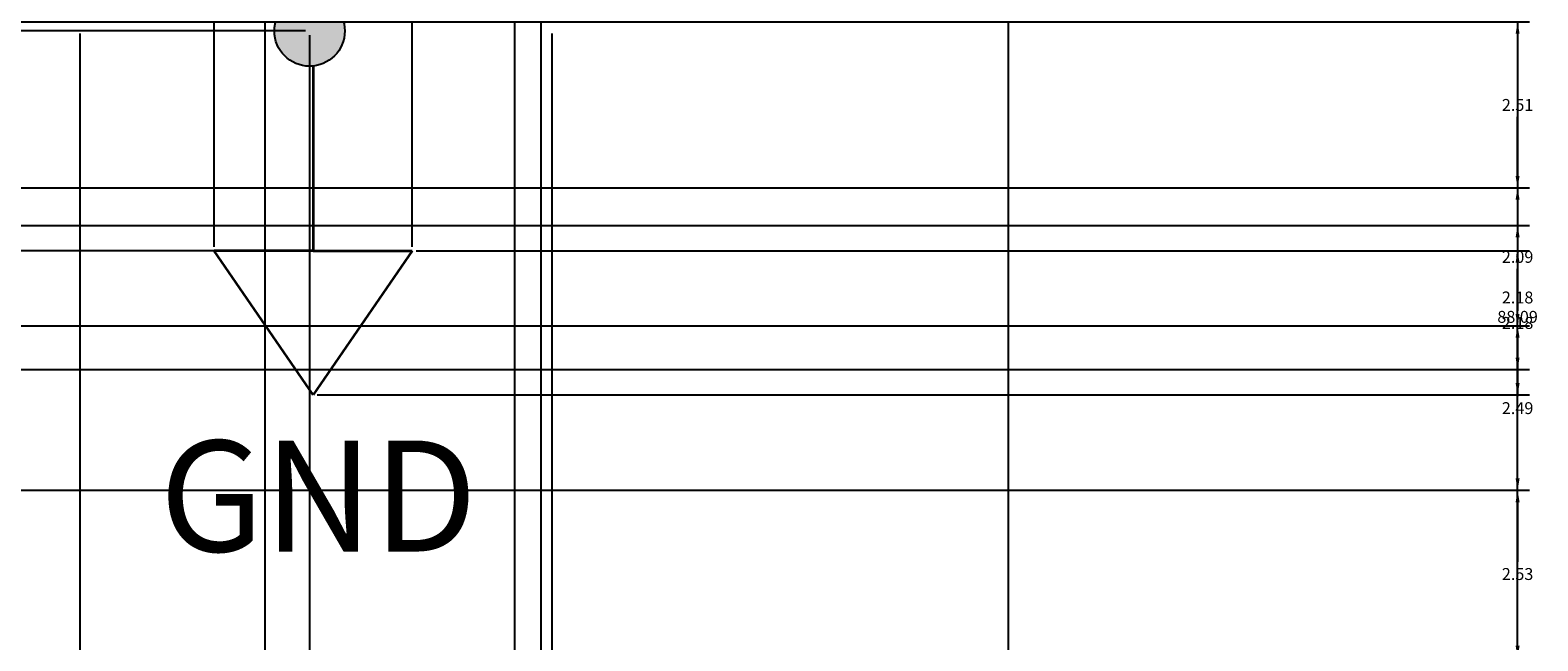
# Model space of a CAD drawing. Units: inches. Extents: x 23 to 132, y 5 to 105.
# Tile 11 of 14: x 106.54 to 129.37, y 50.34 to 59.58. Entities that reach past the tile are written whole.
import ezdxf

# ---------------------------------------------------------------- set-up
doc = ezdxf.new("R2010")
doc.units = ezdxf.units.IN
doc.header["$MEASUREMENT"] = 0
for name, color, linetype, lineweight in [('A-ANNO-DIMS', 2, 'Continuous', 18), ('E-ANNO-IDEN', 4, 'Continuous', 18), ('E-SYMB', 1, 'Continuous', 35), ('E-WIRE', 3, 'Continuous', 25), ('E-WIRE-PATT', 3, 'Continuous', 18)]:
    doc.layers.add(name, color=color, linetype=linetype, lineweight=lineweight)
doc.styles.get("Standard").update_dxf_attribs({"font": 'arial.ttf'})
doc.dimstyles.get("Standard").update_dxf_attribs({"dimtxt": 0.18, "dimasz": 0.18, "dimexe": 0.18, "dimexo": 0.0625, "dimgap": 0.09, "dimtad": 0, "dimtih": 1, "dimtoh": 1, "dimdec": 4, "dimzin": 0, "dimdsep": 46, "dimtxsty": 'Standard', "dimcen": 0.09, "dimadec": 0, "dimazin": 0, "dimtfac": 1, "dimtdec": 4, "dimtofl": 0, "dimtmove": 0, "dimatfit": 3, "dimfxl": 1, "dimtolj": 1, "dimtzin": 0, "dimarcsym": 0})

# ---------------------------------------------------------------- blocks, each defined once
blk = doc.blocks.new('GND')
for p, q in [((1.5, 4.977), (1.5, 2.181)), ((1.5, 2.181), (0, 2.181)), ((1.5, 0), (0, 2.181)), ((1.5, 2.181), (3, 2.181)), ((3, 2.181), (1.5, 0))]:
    blk.add_line(p, q)
blk = doc.blocks.new('*D3')
at = {"layer": 'A-ANNO-DIMS', "color": 0, "lineweight": -2, "transparency": 16777216}
for p, q in [((121.409, 99.285), (129.239, 99.285)), ((129.059, 99.105), (129.059, 55.423)), ((129.059, 11.378), (129.059, 55.06)), ((72.981, 11.198), (129.239, 11.198))]:
    blk.add_line(p, q, dxfattribs=at)
at = {"layer": 'A-ANNO-DIMS', "color": 0, "transparency": 16777216}
for points in [[(129.029, 99.105), (129.089, 99.105), (129.059, 99.285)], [(129.029, 11.378), (129.089, 11.378), (129.059, 11.198)]]:
    blk.add_solid(points, dxfattribs=at)
at = {"layer": 'Defpoints', "color": 0, "transparency": 16777216}
for p in [(121.346, 99.285), (129.059, 99.285), (72.919, 11.198)]:
    blk.add_point(p, dxfattribs=at)
at = {"layer": 'A-ANNO-DIMS', "color": 0, "transparency": 16777216, "insert": (129.059, 55.241), "char_height": 0.18, "attachment_point": 5}
blk.add_mtext('\\A1;88.09', dxfattribs=at)
blk = doc.blocks.new('*D32')
at = {"layer": 'A-ANNO-DIMS', "color": 0, "lineweight": -2, "transparency": 16777216}
for p, q in [((83.576, 59.703), (129.239, 59.703)), ((129.059, 59.523), (129.059, 58.629)), ((129.059, 57.372), (129.059, 58.266)), ((83.576, 57.192), (129.239, 57.192))]:
    blk.add_line(p, q, dxfattribs=at)
at = {"layer": 'A-ANNO-DIMS', "color": 0, "transparency": 16777216}
for points in [[(129.029, 59.523), (129.089, 59.523), (129.059, 59.703)], [(129.029, 57.372), (129.089, 57.372), (129.059, 57.192)]]:
    blk.add_solid(points, dxfattribs=at)
at = {"layer": 'Defpoints', "color": 0, "transparency": 16777216}
for p in [(83.514, 59.703), (83.514, 57.192), (129.059, 57.192)]:
    blk.add_point(p, dxfattribs=at)
at = {"layer": 'A-ANNO-DIMS', "color": 0, "transparency": 16777216, "insert": (129.059, 58.447), "char_height": 0.18, "attachment_point": 5}
blk.add_mtext('\\A1;2.51', dxfattribs=at)
blk = doc.blocks.new('*D33')
at = {"layer": 'A-ANNO-DIMS', "color": 0, "lineweight": -2, "transparency": 16777216}
for p, q in [((83.576, 57.192), (129.239, 57.192)), ((129.059, 57.012), (129.059, 56.33)), ((129.059, 55.284), (129.059, 55.966)), ((83.576, 55.104), (129.239, 55.104))]:
    blk.add_line(p, q, dxfattribs=at)
at = {"layer": 'A-ANNO-DIMS', "color": 0, "transparency": 16777216}
for points in [[(129.029, 57.012), (129.089, 57.012), (129.059, 57.192)], [(129.029, 55.284), (129.089, 55.284), (129.059, 55.104)]]:
    blk.add_solid(points, dxfattribs=at)
at = {"layer": 'Defpoints', "color": 0, "transparency": 16777216}
for p in [(83.514, 57.192), (83.514, 55.104), (129.059, 55.104)]:
    blk.add_point(p, dxfattribs=at)
at = {"layer": 'A-ANNO-DIMS', "color": 0, "transparency": 16777216, "insert": (129.059, 56.148), "char_height": 0.18, "attachment_point": 5}
blk.add_mtext('\\A1;2.09', dxfattribs=at)
blk = doc.blocks.new('*D34')
at = {"layer": 'A-ANNO-DIMS', "color": 0, "lineweight": -2, "transparency": 16777216}
for p, q in [((83.576, 55.104), (129.239, 55.104)), ((129.059, 54.924), (129.059, 54.042)), ((129.059, 52.797), (129.059, 53.678)), ((83.576, 52.617), (129.239, 52.617))]:
    blk.add_line(p, q, dxfattribs=at)
at = {"layer": 'A-ANNO-DIMS', "color": 0, "transparency": 16777216}
for points in [[(129.029, 54.924), (129.089, 54.924), (129.059, 55.104)], [(129.029, 52.797), (129.089, 52.797), (129.059, 52.617)]]:
    blk.add_solid(points, dxfattribs=at)
at = {"layer": 'Defpoints', "color": 0, "transparency": 16777216}
for p in [(83.514, 55.104), (83.514, 52.617), (129.059, 52.617)]:
    blk.add_point(p, dxfattribs=at)
at = {"layer": 'A-ANNO-DIMS', "color": 0, "transparency": 16777216, "insert": (129.059, 53.86), "char_height": 0.18, "attachment_point": 5}
blk.add_mtext('\\A1;2.49', dxfattribs=at)
blk = doc.blocks.new('*D35')
at = {"layer": 'A-ANNO-DIMS', "color": 0, "lineweight": -2, "transparency": 16777216}
for p, q in [((83.576, 52.617), (129.239, 52.617)), ((129.059, 52.437), (129.059, 51.532)), ((129.059, 50.264), (129.059, 51.168)), ((83.576, 50.084), (129.239, 50.084))]:
    blk.add_line(p, q, dxfattribs=at)
at = {"layer": 'A-ANNO-DIMS', "color": 0, "transparency": 16777216}
for points in [[(129.029, 52.437), (129.089, 52.437), (129.059, 52.617)], [(129.029, 50.264), (129.089, 50.264), (129.059, 50.084)]]:
    blk.add_solid(points, dxfattribs=at)
at = {"layer": 'Defpoints', "color": 0, "transparency": 16777216}
for p in [(83.514, 52.617), (83.514, 50.084), (129.059, 50.084)]:
    blk.add_point(p, dxfattribs=at)
at = {"layer": 'A-ANNO-DIMS', "color": 0, "transparency": 16777216, "insert": (129.059, 51.35), "char_height": 0.18, "attachment_point": 5}
blk.add_mtext('\\A1;2.53', dxfattribs=at)
blk = doc.blocks.new('*D70')
at = {"layer": 'A-ANNO-DIMS', "color": 0, "lineweight": -2, "transparency": 16777216}
for p, q in [((35.392, 56.625), (129.239, 56.625)), ((129.059, 56.445), (129.059, 55.716)), ((129.059, 54.624), (129.059, 55.352)), ((33.892, 54.444), (129.239, 54.444))]:
    blk.add_line(p, q, dxfattribs=at)
at = {"layer": 'A-ANNO-DIMS', "color": 0, "transparency": 16777216}
for points in [[(129.029, 56.445), (129.089, 56.445), (129.059, 56.625)], [(129.029, 54.624), (129.089, 54.624), (129.059, 54.444)]]:
    blk.add_solid(points, dxfattribs=at)
at = {"layer": 'Defpoints', "color": 0, "transparency": 16777216}
for p in [(35.33, 56.625), (33.83, 54.444), (129.059, 54.444)]:
    blk.add_point(p, dxfattribs=at)
at = {"layer": 'A-ANNO-DIMS', "color": 0, "transparency": 16777216, "insert": (129.059, 55.534), "char_height": 0.18, "attachment_point": 5}
blk.add_mtext('\\A1;2.18', dxfattribs=at)
blk = doc.blocks.new('*D75')
at = {"layer": 'A-ANNO-DIMS', "color": 0, "lineweight": -2, "transparency": 16777216}
for p, q in [((107.287, 59.528), (107.287, 5.443)), ((110.768, 59.503), (110.768, 5.443)), ((107.467, 5.623), (108.704, 5.623)), ((110.588, 5.623), (109.351, 5.623))]:
    blk.add_line(p, q, dxfattribs=at)
at = {"layer": 'A-ANNO-DIMS', "color": 0, "transparency": 16777216}
for points in [[(107.467, 5.653), (107.467, 5.593), (107.287, 5.623)], [(110.588, 5.653), (110.588, 5.593), (110.768, 5.623)]]:
    blk.add_solid(points, dxfattribs=at)
at = {"layer": 'Defpoints', "color": 0, "transparency": 16777216}
for p in [(107.287, 59.59), (110.768, 59.566), (110.768, 5.623)]:
    blk.add_point(p, dxfattribs=at)
at = {"layer": 'A-ANNO-DIMS', "color": 0, "transparency": 16777216, "insert": (109.028, 5.623), "char_height": 0.18, "attachment_point": 5}
blk.add_mtext('\\A1;3.48', dxfattribs=at)
blk = doc.blocks.new('*D76')
at = {"layer": 'A-ANNO-DIMS', "color": 0, "lineweight": -2, "transparency": 16777216}
for p, q in [((110.768, 59.503), (110.768, 5.443)), ((114.434, 59.528), (114.434, 5.443)), ((110.948, 5.623), (112.207, 5.623)), ((114.254, 5.623), (112.994, 5.623))]:
    blk.add_line(p, q, dxfattribs=at)
at = {"layer": 'A-ANNO-DIMS', "color": 0, "transparency": 16777216}
for points in [[(110.948, 5.653), (110.948, 5.593), (110.768, 5.623)], [(114.254, 5.653), (114.254, 5.593), (114.434, 5.623)]]:
    blk.add_solid(points, dxfattribs=at)
at = {"layer": 'Defpoints', "color": 0, "transparency": 16777216}
for p in [(114.434, 59.59), (110.768, 59.566), (114.434, 5.623)]:
    blk.add_point(p, dxfattribs=at)
at = {"layer": 'A-ANNO-DIMS', "color": 0, "transparency": 16777216, "insert": (112.601, 5.623), "char_height": 0.18, "attachment_point": 5}
blk.add_mtext('\\A1;3.666', dxfattribs=at)
blk = doc.blocks.new('*D81')
at = {"layer": 'A-ANNO-DIMS', "color": 0, "lineweight": -2, "transparency": 16777216}
for p, q in [((110.705, 59.566), (22.942, 59.566)), ((23.122, 59.386), (23.122, 58.085)), ((23.122, 56.42), (23.122, 57.721)), ((110.759, 56.24), (22.942, 56.24))]:
    blk.add_line(p, q, dxfattribs=at)
at = {"layer": 'A-ANNO-DIMS', "color": 0, "transparency": 16777216}
for points in [[(23.092, 59.386), (23.152, 59.386), (23.122, 59.566)], [(23.092, 56.42), (23.152, 56.42), (23.122, 56.24)]]:
    blk.add_solid(points, dxfattribs=at)
at = {"layer": 'Defpoints', "color": 0, "transparency": 16777216}
for p in [(23.122, 59.566), (110.768, 59.566), (110.822, 56.24)]:
    blk.add_point(p, dxfattribs=at)
at = {"layer": 'A-ANNO-DIMS', "color": 0, "transparency": 16777216, "insert": (23.122, 57.903), "char_height": 0.18, "attachment_point": 5}
blk.add_mtext('\\A1;3.326', dxfattribs=at)
blk = doc.blocks.new('*D82')
at = {"layer": 'A-ANNO-DIMS', "color": 0, "lineweight": -2, "transparency": 16777216}
for p, q in [((109.322, 56.302), (109.322, 105.232)), ((109.502, 105.052), (110.673, 105.052)), ((112.142, 105.052), (110.971, 105.052)), ((112.322, 56.302), (112.322, 105.232))]:
    blk.add_line(p, q, dxfattribs=at)
at = {"layer": 'A-ANNO-DIMS', "color": 0, "transparency": 16777216}
for points in [[(109.502, 105.082), (109.502, 105.022), (109.322, 105.052)], [(112.142, 105.082), (112.142, 105.022), (112.322, 105.052)]]:
    blk.add_solid(points, dxfattribs=at)
at = {"layer": 'Defpoints', "color": 0, "transparency": 16777216}
for p in [(112.322, 105.052), (109.322, 56.24), (112.322, 56.24)]:
    blk.add_point(p, dxfattribs=at)
at = {"layer": 'A-ANNO-DIMS', "color": 0, "transparency": 16777216, "insert": (110.822, 105.052), "char_height": 0.18, "attachment_point": 5}
blk.add_mtext('\\A1;3', dxfattribs=at)
blk = doc.blocks.new('*D83')
at = {"layer": 'A-ANNO-DIMS', "color": 0, "lineweight": -2, "transparency": 16777216}
for p, q in [((112.384, 56.24), (129.239, 56.24)), ((129.059, 56.06), (129.059, 55.331)), ((129.059, 54.239), (129.059, 54.967)), ((110.884, 54.059), (129.239, 54.059))]:
    blk.add_line(p, q, dxfattribs=at)
at = {"layer": 'A-ANNO-DIMS', "color": 0, "transparency": 16777216}
for points in [[(129.029, 56.06), (129.089, 56.06), (129.059, 56.24)], [(129.029, 54.239), (129.089, 54.239), (129.059, 54.059)]]:
    blk.add_solid(points, dxfattribs=at)
at = {"layer": 'Defpoints', "color": 0, "transparency": 16777216}
for p in [(112.322, 56.24), (110.822, 54.059), (129.059, 54.059)]:
    blk.add_point(p, dxfattribs=at)
at = {"layer": 'A-ANNO-DIMS', "color": 0, "transparency": 16777216, "insert": (129.059, 55.149), "char_height": 0.18, "attachment_point": 5}
blk.add_mtext('\\A1;2.18', dxfattribs=at)
blk = doc.blocks.new('*D91')
at = {"layer": 'A-ANNO-DIMS', "color": 0, "lineweight": -2, "transparency": 16777216}
for p, q in [((110.089, 79.853), (110.089, 5.443)), ((113.872, 79.853), (113.872, 5.443)), ((110.269, 5.623), (111.587, 5.623)), ((113.692, 5.623), (112.374, 5.623))]:
    blk.add_line(p, q, dxfattribs=at)
at = {"layer": 'A-ANNO-DIMS', "color": 0, "transparency": 16777216}
for points in [[(110.269, 5.653), (110.269, 5.593), (110.089, 5.623)], [(113.692, 5.653), (113.692, 5.593), (113.872, 5.623)]]:
    blk.add_solid(points, dxfattribs=at)
at = {"layer": 'Defpoints', "color": 0, "transparency": 16777216}
for p in [(110.089, 79.916), (113.872, 79.916), (113.872, 5.623)]:
    blk.add_point(p, dxfattribs=at)
at = {"layer": 'A-ANNO-DIMS', "color": 0, "transparency": 16777216, "insert": (111.981, 5.623), "char_height": 0.18, "attachment_point": 5}
blk.add_mtext('\\A1;3.783', dxfattribs=at)
blk = doc.blocks.new('*D93')
at = {"layer": 'A-ANNO-DIMS', "color": 0, "lineweight": -2, "transparency": 16777216}
for p, q in [((114.269, 94.721), (114.269, 5.443)), ((121.346, 94.721), (121.346, 5.443)), ((114.449, 5.623), (117.415, 5.623)), ((121.166, 5.623), (118.201, 5.623))]:
    blk.add_line(p, q, dxfattribs=at)
at = {"layer": 'A-ANNO-DIMS', "color": 0, "transparency": 16777216}
for points in [[(114.449, 5.653), (114.449, 5.593), (114.269, 5.623)], [(121.166, 5.653), (121.166, 5.593), (121.346, 5.623)]]:
    blk.add_solid(points, dxfattribs=at)
at = {"layer": 'Defpoints', "color": 0, "transparency": 16777216}
for p in [(114.269, 94.783), (121.346, 94.783), (121.346, 5.623)]:
    blk.add_point(p, dxfattribs=at)
at = {"layer": 'A-ANNO-DIMS', "color": 0, "transparency": 16777216, "insert": (117.808, 5.623), "char_height": 0.18, "attachment_point": 5}
blk.add_mtext('\\A1;7.077', dxfattribs=at)

msp = doc.modelspace()

# ---------------------------------------------------------------- hatches: boundary and pattern name
at = {"layer": 'E-WIRE-PATT'}
h = msp.add_hatch(color=256, dxfattribs=at)
h.dxf.hatch_style = 1
h.paths.add_polyline_path([(107.8201, 73.3945, 0.4142136), (107.2874, 73.9273), (107.2874, 72.8618, 0.4142136)])
h.paths.add_polyline_path([(107.2874, 73.9273, 0.4142136), (106.7546, 73.3945, 0.4142136), (107.2874, 72.8618)])
h.paths.add_polyline_path([(110.2355, 59.5904), (111.2999, 59.5904, 0.9551697)])
h.paths.add_polyline_path([(111.3005, 59.566, 0.011463), (111.2999, 59.5904), (110.2355, 59.5904, 0.011463), (110.235, 59.566, 1)])

# ---------------------------------------------------------------- linework, layer by layer
at = {"layer": 'E-WIRE'}
msp.add_circle((110.7677, 59.566), 0.5327, dxfattribs=at)

# ---------------------------------------------------------------- block references
at = {"layer": 'E-SYMB'}
msp.add_blockref('GND', (109.322, 54.059), dxfattribs=at)

# ---------------------------------------------------------------- texts
at = {"layer": 'E-ANNO-IDEN'}
msp.add_text('GND', height=1.67943, dxfattribs=at).set_placement((108.4964, 51.6894))

# ---------------------------------------------------------------- dimensions: what is measured, and where the dimension line sits
at = {"layer": 'A-ANNO-DIMS'}
for base, p1, p2, override, picture, middle in [((112.3219, 105.052), (109.3219, 56.2399), (112.3219, 56.2399), {"dimdec": 0, "dimlfac": 1, "dimrnd": 0, "dimzin": 0, "dimdsep": 46, "dimlunit": 2}, '*D82', (110.8219, 105.052)), ((121.3461, 5.6233), (114.2693, 94.7833), (121.3461, 94.7833), {"dimdec": 3, "dimlfac": 1, "dimrnd": 0, "dimzin": 0, "dimdsep": 46, "dimlunit": 2}, '*D93', (117.8077, 5.6233)), ((113.8719, 5.6233), (110.0892, 79.9158), (113.8719, 79.9158), {"dimdec": 3, "dimlfac": 1, "dimrnd": 0, "dimzin": 0, "dimdsep": 46, "dimlunit": 2}, '*D91', (111.9805, 5.6233)), ((110.7677, 5.6233), (107.2874, 59.5904), (110.7677, 59.566), {"dimdec": 2, "dimlfac": 1, "dimrnd": 0, "dimzin": 0, "dimdsep": 46, "dimlunit": 2}, '*D75', (109.0275, 5.6233)), ((114.434, 5.6233), (110.7677, 59.566), (114.434, 59.5904), {"dimdec": 3, "dimlfac": 1, "dimrnd": 0, "dimzin": 0, "dimdsep": 46, "dimlunit": 2}, '*D76', (112.6009, 5.6233))]:
    dim = msp.add_linear_dim(base=base, p1=p1, p2=p2, dimstyle='Standard', override=override, dxfattribs=at)
    dim.commit()
    dim.dimension.update_dxf_attribs({"geometry": picture, "text_midpoint": middle})
for base, p1, p2, override, picture, middle in [((129.0589, 99.2846), (72.9188, 11.1983), (121.3461, 99.2846), {"dimdec": 2, "dimlfac": 1, "dimrnd": 0, "dimzin": 0, "dimdsep": 46, "dimlunit": 2}, '*D3', (129.0589, 55.2415)), ((129.0589, 57.1918), (83.5136, 59.7032), (83.5136, 57.1918), {"dimdec": 2, "dimlfac": 1, "dimrnd": 0, "dimzin": 0, "dimdsep": 46, "dimlunit": 2}, '*D32', (129.0589, 58.4475)), ((23.1215, 59.566), (110.8219, 56.2399), (110.7677, 59.566), {"dimdec": 3, "dimlfac": 1, "dimrnd": 0, "dimzin": 0, "dimdsep": 46, "dimlunit": 2}, '*D81', (23.1215, 57.9029)), ((129.0589, 55.1036), (83.5136, 57.1918), (83.5136, 55.1036), {"dimdec": 2, "dimlfac": 1, "dimrnd": 0, "dimzin": 0, "dimdsep": 46, "dimlunit": 2}, '*D33', (129.0589, 56.1477)), ((129.0589, 54.4437), (35.3299, 56.6249), (33.8299, 54.4437), {"dimdec": 2, "dimlfac": 1, "dimrnd": 0, "dimzin": 0, "dimdsep": 46, "dimlunit": 2}, '*D70', (129.0589, 55.5343)), ((129.0589, 54.0586), (112.3219, 56.2399), (110.8219, 54.0586), {"dimdec": 2, "dimlfac": 1, "dimrnd": 0, "dimzin": 0, "dimdsep": 46, "dimlunit": 2}, '*D83', (129.0589, 55.1492)), ((129.0589, 52.6172), (83.5136, 55.1036), (83.5136, 52.6172), {"dimdec": 2, "dimlfac": 1, "dimrnd": 0, "dimzin": 0, "dimdsep": 46, "dimlunit": 2}, '*D34', (129.0589, 53.8604)), ((129.0589, 50.0837), (83.5136, 52.6172), (83.5136, 50.0837), {"dimdec": 2, "dimlfac": 1, "dimrnd": 0, "dimzin": 0, "dimdsep": 46, "dimlunit": 2}, '*D35', (129.0589, 51.3504))]:
    dim = msp.add_linear_dim(base=base, p1=p1, p2=p2, angle=90, dimstyle='Standard', override=override, dxfattribs=at)
    dim.commit()
    dim.dimension.update_dxf_attribs({"geometry": picture, "text_midpoint": middle})

doc.saveas('drawing.dxf')
